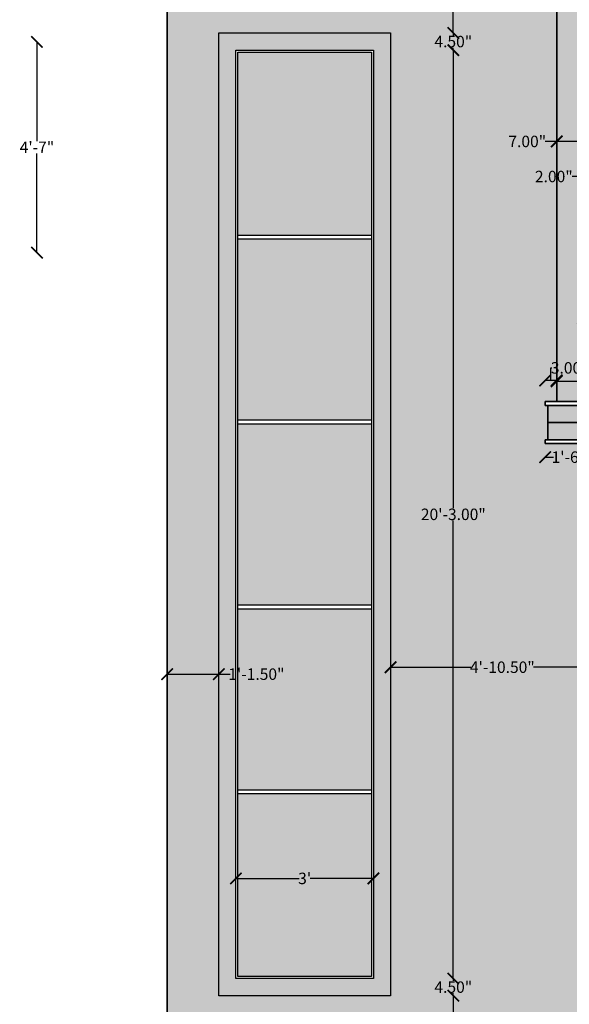
# Model space of a CAD drawing. Units: inches. Extents: x -654 to 390, y -40 to 648.
# Tile 5 of 13: x -40 to 104, y 159 to 417. Entities that reach past the tile are written whole.
import ezdxf

# ---------------------------------------------------------------- set-up
doc = ezdxf.new("R2010")
doc.units = ezdxf.units.IN
doc.header["$PDMODE"] = 3
for name, color, linetype, lineweight in [('A-ANNO-DIMS', 2, 'Continuous', 18), ('A-ELEV', 7, 'Continuous', 35), ('A-ELEV-FILL', 252, 'Continuous', 13), ('A-ELEV-PATT', 8, 'Continuous', 13), ('A-GLAZ', 4, 'Continuous', 25)]:
    doc.layers.add(name, color=color, linetype=linetype, lineweight=lineweight)
doc.styles.get("Standard").update_dxf_attribs({"font": 'arial.ttf'})
doc.dimstyles.get("Standard").update_dxf_attribs({"dimtxt": 3, "dimasz": 3, "dimexe": 0.18, "dimexo": 0.0625, "dimgap": 0.09, "dimtad": 0, "dimtih": 1, "dimtoh": 1, "dimzin": 0, "dimdsep": 46, "dimlunit": 3, "dimtxsty": 'Standard', "dimblk": 'ARCHTICK', "dimcen": 0.09, "dimse1": 1, "dimse2": 1, "dimadec": 0, "dimazin": 0, "dimtfac": 1, "dimtofl": 0, "dimtmove": 0, "dimatfit": 3, "dimfxl": 1, "dimtolj": 1, "dimtzin": 0, "dimarcsym": 0})

# ---------------------------------------------------------------- blocks, each defined once
blk = doc.blocks.new('_ArchTick')
at = {"color": 0, "linetype": 'ByBlock', "const_width": 0.15}
blk.add_lwpolyline([(-0.5, -0.5), (0.5, 0.5)], dxfattribs=at)
blk = doc.blocks.new('*D20')
at = {"layer": 'A-ANNO-DIMS', "color": 0, "lineweight": -2, "transparency": 16777216}
for p, q in [((73.57, 442.63), (73.57, 429.51)), ((73.57, 413.13), (73.57, 426.26))]:
    blk.add_line(p, q, dxfattribs=at)
at = {"layer": 'Defpoints', "color": 0, "transparency": 16777216}
for p in [(73.57, 442.63), (57.15, 413.13), (73.57, 413.13)]:
    blk.add_point(p, dxfattribs=at)
at = {"layer": 'A-ANNO-DIMS', "color": 0, "lineweight": -2, "transparency": 16777216, "xscale": 3, "yscale": 3, "zscale": 3}
for p, rotation in [((73.57, 442.63), 90), ((73.57, 413.13), 270)]:
    blk.add_blockref('_ArchTick', p, dxfattribs=dict(at, rotation=rotation))
at = {"layer": 'A-ANNO-DIMS', "color": 0, "transparency": 16777216, "insert": (73.57, 427.88), "char_height": 3, "attachment_point": 5}
blk.add_mtext('\\A1;2\'-5.50"', dxfattribs=at)
blk = doc.blocks.new('*D21')
at = {"layer": 'A-ANNO-DIMS', "color": 0, "lineweight": -2, "transparency": 16777216}
for p, q in [((73.57, 413.13), (73.57, 412.51)), ((73.57, 408.63), (73.57, 409.26))]:
    blk.add_line(p, q, dxfattribs=at)
at = {"layer": 'Defpoints', "color": 0, "transparency": 16777216}
for p in [(57.15, 413.13), (52.65, 408.63), (73.57, 408.63)]:
    blk.add_point(p, dxfattribs=at)
at = {"layer": 'A-ANNO-DIMS', "color": 0, "lineweight": -2, "transparency": 16777216, "xscale": 3, "yscale": 3, "zscale": 3}
for p, rotation in [((73.57, 413.13), 90), ((73.57, 408.63), 270)]:
    blk.add_blockref('_ArchTick', p, dxfattribs=dict(at, rotation=rotation))
at = {"layer": 'A-ANNO-DIMS', "color": 0, "transparency": 16777216, "insert": (73.57, 410.88), "char_height": 3, "attachment_point": 5}
blk.add_mtext('\\A1;4.50"', dxfattribs=at)
blk = doc.blocks.new('*D22')
at = {"layer": 'A-ANNO-DIMS', "color": 0, "lineweight": -2, "transparency": 16777216}
for p, q in [((73.57, 408.63), (73.57, 288.76)), ((73.57, 165.63), (73.57, 285.51))]:
    blk.add_line(p, q, dxfattribs=at)
at = {"layer": 'Defpoints', "color": 0, "transparency": 16777216}
for p in [(52.65, 408.63), (52.65, 165.63), (73.57, 165.63)]:
    blk.add_point(p, dxfattribs=at)
at = {"layer": 'A-ANNO-DIMS', "color": 0, "lineweight": -2, "transparency": 16777216, "xscale": 3, "yscale": 3, "zscale": 3}
for p, rotation in [((73.57, 408.63), 90), ((73.57, 165.63), 270)]:
    blk.add_blockref('_ArchTick', p, dxfattribs=dict(at, rotation=rotation))
at = {"layer": 'A-ANNO-DIMS', "color": 0, "transparency": 16777216, "insert": (73.57, 287.13), "char_height": 3, "attachment_point": 5}
blk.add_mtext('\\A1;20\'-3.00"', dxfattribs=at)
blk = doc.blocks.new('*D23')
at = {"layer": 'A-ANNO-DIMS', "color": 0, "lineweight": -2, "transparency": 16777216}
for p, q in [((73.57, 165.63), (73.57, 165.01)), ((73.57, 161.13), (73.57, 161.76))]:
    blk.add_line(p, q, dxfattribs=at)
at = {"layer": 'Defpoints', "color": 0, "transparency": 16777216}
for p in [(52.65, 165.63), (57.15, 161.13), (73.57, 161.13)]:
    blk.add_point(p, dxfattribs=at)
at = {"layer": 'A-ANNO-DIMS', "color": 0, "lineweight": -2, "transparency": 16777216, "xscale": 3, "yscale": 3, "zscale": 3}
for p, rotation in [((73.57, 165.63), 90), ((73.57, 161.13), 270)]:
    blk.add_blockref('_ArchTick', p, dxfattribs=dict(at, rotation=rotation))
at = {"layer": 'A-ANNO-DIMS', "color": 0, "transparency": 16777216, "insert": (73.57, 163.38), "char_height": 3, "attachment_point": 5}
blk.add_mtext('\\A1;4.50"', dxfattribs=at)
blk = doc.blocks.new('*D24')
at = {"layer": 'A-ANNO-DIMS', "color": 0, "lineweight": -2, "transparency": 16777216}
for p, q in [((73.57, 161.13), (73.57, 144.76)), ((73.57, 125.13), (73.57, 141.51))]:
    blk.add_line(p, q, dxfattribs=at)
at = {"layer": 'Defpoints', "color": 0, "transparency": 16777216}
for p in [(57.15, 161.13), (73.57, 125.13), (73.57, 125.13)]:
    blk.add_point(p, dxfattribs=at)
at = {"layer": 'A-ANNO-DIMS', "color": 0, "lineweight": -2, "transparency": 16777216, "xscale": 3, "yscale": 3, "zscale": 3}
for p, rotation in [((73.57, 161.13), 90), ((73.57, 125.13), 270)]:
    blk.add_blockref('_ArchTick', p, dxfattribs=dict(at, rotation=rotation))
at = {"layer": 'A-ANNO-DIMS', "color": 0, "transparency": 16777216, "insert": (73.57, 143.13), "char_height": 3, "attachment_point": 5}
blk.add_mtext("\\A1;3'", dxfattribs=at)
blk = doc.blocks.new('*D45')
at = {"layer": 'A-ANNO-DIMS', "color": 0, "lineweight": -2, "transparency": 16777216}
for p, q in [((99.15, 322.17), (99.15, 325.47)), ((99.15, 325.47), (99.33, 325.47)), ((100.65, 322.17), (97.65, 322.17))]:
    blk.add_line(p, q, dxfattribs=at)
at = {"layer": 'Defpoints', "color": 0, "transparency": 16777216}
for p in [(97.65, 322.17), (97.65, 316.63), (100.65, 316.63)]:
    blk.add_point(p, dxfattribs=at)
at = {"layer": 'A-ANNO-DIMS', "color": 0, "lineweight": -2, "transparency": 16777216, "xscale": 3, "yscale": 3, "zscale": 3, "rotation": 180}
blk.add_blockref('_ArchTick', (97.65, 322.17), dxfattribs=at)
at = {"layer": 'A-ANNO-DIMS', "color": 0, "lineweight": -2, "transparency": 16777216, "xscale": 3, "yscale": 3, "zscale": 3}
blk.add_blockref('_ArchTick', (100.65, 322.17), dxfattribs=at)
at = {"layer": 'A-ANNO-DIMS', "color": 0, "transparency": 16777216, "insert": (104.05, 325.47), "char_height": 3, "attachment_point": 5}
blk.add_mtext('\\A1;3.00"', dxfattribs=at)
blk = doc.blocks.new('*D47')
at = {"layer": 'A-ANNO-DIMS', "color": 0, "lineweight": -2, "transparency": 16777216}
for p, q in [((100.65, 321.96), (116.16, 321.96)), ((145.65, 321.96), (130.14, 321.96))]:
    blk.add_line(p, q, dxfattribs=at)
at = {"layer": 'Defpoints', "color": 0, "transparency": 16777216}
for p in [(145.65, 329.63), (100.65, 322.17), (100.65, 321.96)]:
    blk.add_point(p, dxfattribs=at)
at = {"layer": 'A-ANNO-DIMS', "color": 0, "lineweight": -2, "transparency": 16777216, "xscale": 3, "yscale": 3, "zscale": 3, "rotation": 180}
blk.add_blockref('_ArchTick', (100.65, 321.96), dxfattribs=at)
at = {"layer": 'A-ANNO-DIMS', "color": 0, "lineweight": -2, "transparency": 16777216, "xscale": 3, "yscale": 3, "zscale": 3}
blk.add_blockref('_ArchTick', (145.65, 321.96), dxfattribs=at)
at = {"layer": 'A-ANNO-DIMS', "color": 0, "transparency": 16777216, "insert": (123.15, 321.96), "char_height": 3, "attachment_point": 5}
blk.add_mtext('\\A1;3\'-9.00"', dxfattribs=at)
blk = doc.blocks.new('*D48')
at = {"layer": 'A-ANNO-DIMS', "color": 0, "lineweight": -2, "transparency": 16777216}
for p, q in [((113.1, 359.63), (113.1, 339.76)), ((113.1, 316.63), (113.1, 336.51))]:
    blk.add_line(p, q, dxfattribs=at)
at = {"layer": 'Defpoints', "color": 0, "transparency": 16777216}
for p in [(107.65, 359.63), (113.1, 359.63), (100.65, 316.63)]:
    blk.add_point(p, dxfattribs=at)
at = {"layer": 'A-ANNO-DIMS', "color": 0, "lineweight": -2, "transparency": 16777216, "xscale": 3, "yscale": 3, "zscale": 3}
for p, rotation in [((113.1, 359.63), 90), ((113.1, 316.63), 270)]:
    blk.add_blockref('_ArchTick', p, dxfattribs=dict(at, rotation=rotation))
at = {"layer": 'A-ANNO-DIMS', "color": 0, "transparency": 16777216, "insert": (113.1, 338.13), "char_height": 3, "attachment_point": 5}
blk.add_mtext('\\A1;3\'-7.00"', dxfattribs=at)
blk = doc.blocks.new('*D53')
at = {"layer": 'A-ANNO-DIMS', "color": 0, "lineweight": -2, "transparency": 16777216}
for p, q in [((100.65, 384.74), (97.65, 384.74)), ((107.65, 384.74), (100.65, 384.74))]:
    blk.add_line(p, q, dxfattribs=at)
at = {"layer": 'Defpoints', "color": 0, "transparency": 16777216}
for p in [(100.65, 384.74), (100.65, 359.63), (107.65, 359.63)]:
    blk.add_point(p, dxfattribs=at)
at = {"layer": 'A-ANNO-DIMS', "color": 0, "lineweight": -2, "transparency": 16777216, "xscale": 3, "yscale": 3, "zscale": 3, "rotation": 180}
blk.add_blockref('_ArchTick', (100.65, 384.74), dxfattribs=at)
at = {"layer": 'A-ANNO-DIMS', "color": 0, "lineweight": -2, "transparency": 16777216, "xscale": 3, "yscale": 3, "zscale": 3}
blk.add_blockref('_ArchTick', (107.65, 384.74), dxfattribs=at)
at = {"layer": 'A-ANNO-DIMS', "color": 0, "transparency": 16777216, "insert": (92.93, 384.74), "char_height": 3, "attachment_point": 5}
blk.add_mtext('\\A1;7.00"', dxfattribs=at)
blk = doc.blocks.new('*D54')
at = {"layer": 'A-ANNO-DIMS', "color": 0, "lineweight": -2, "transparency": 16777216}
for p, q in [((107.65, 375.56), (104.65, 375.56)), ((109.65, 375.56), (107.65, 375.56))]:
    blk.add_line(p, q, dxfattribs=at)
at = {"layer": 'Defpoints', "color": 0, "transparency": 16777216}
for p in [(107.65, 375.56), (107.65, 361.63), (109.65, 361.63)]:
    blk.add_point(p, dxfattribs=at)
at = {"layer": 'A-ANNO-DIMS', "color": 0, "lineweight": -2, "transparency": 16777216, "xscale": 3, "yscale": 3, "zscale": 3, "rotation": 180}
blk.add_blockref('_ArchTick', (107.65, 375.56), dxfattribs=at)
at = {"layer": 'A-ANNO-DIMS', "color": 0, "lineweight": -2, "transparency": 16777216, "xscale": 3, "yscale": 3, "zscale": 3}
blk.add_blockref('_ArchTick', (109.65, 375.56), dxfattribs=at)
at = {"layer": 'A-ANNO-DIMS', "color": 0, "transparency": 16777216, "insert": (99.89, 375.56), "char_height": 3, "attachment_point": 5}
blk.add_mtext('\\A1;2.00"', dxfattribs=at)
blk = doc.blocks.new('*D65')
at = {"layer": 'A-ANNO-DIMS', "color": 0, "lineweight": -2, "transparency": 16777216}
for p, q in [((-1.35, 245.3), (12.15, 245.3)), ((12.15, 245.3), (15.15, 245.3))]:
    blk.add_line(p, q, dxfattribs=at)
at = {"layer": 'Defpoints', "color": 0, "transparency": 16777216}
for p in [(12.15, 245.3), (12.15, 161.13), (-1.35, 125.13)]:
    blk.add_point(p, dxfattribs=at)
at = {"layer": 'A-ANNO-DIMS', "color": 0, "lineweight": -2, "transparency": 16777216, "xscale": 3, "yscale": 3, "zscale": 3, "rotation": 180}
blk.add_blockref('_ArchTick', (-1.35, 245.3), dxfattribs=at)
at = {"layer": 'A-ANNO-DIMS', "color": 0, "lineweight": -2, "transparency": 16777216, "xscale": 3, "yscale": 3, "zscale": 3}
blk.add_blockref('_ArchTick', (12.15, 245.3), dxfattribs=at)
at = {"layer": 'A-ANNO-DIMS', "color": 0, "transparency": 16777216, "insert": (22, 245.3), "char_height": 3, "attachment_point": 5}
blk.add_mtext('\\A1;1\'-1.50"', dxfattribs=at)
blk = doc.blocks.new('*D66')
at = {"layer": 'A-ANNO-DIMS', "color": 0, "lineweight": -2, "transparency": 16777216}
for p, q in [((16.65, 191.84), (33.18, 191.84)), ((52.65, 191.84), (36.12, 191.84))]:
    blk.add_line(p, q, dxfattribs=at)
at = {"layer": 'Defpoints', "color": 0, "transparency": 16777216}
for p in [(52.65, 191.84), (16.65, 165.63), (52.65, 165.63)]:
    blk.add_point(p, dxfattribs=at)
at = {"layer": 'A-ANNO-DIMS', "color": 0, "lineweight": -2, "transparency": 16777216, "xscale": 3, "yscale": 3, "zscale": 3, "rotation": 180}
blk.add_blockref('_ArchTick', (16.65, 191.84), dxfattribs=at)
at = {"layer": 'A-ANNO-DIMS', "color": 0, "lineweight": -2, "transparency": 16777216, "xscale": 3, "yscale": 3, "zscale": 3}
blk.add_blockref('_ArchTick', (52.65, 191.84), dxfattribs=at)
at = {"layer": 'A-ANNO-DIMS', "color": 0, "transparency": 16777216, "insert": (34.65, 191.84), "char_height": 3, "attachment_point": 5}
blk.add_mtext("\\A1;3'", dxfattribs=at)
blk = doc.blocks.new('*D67')
at = {"layer": 'A-ANNO-DIMS', "color": 0, "lineweight": -2, "transparency": 16777216}
for p, q in [((52.65, 153.11), (57.15, 153.11)), ((57.15, 153.11), (60.15, 153.11))]:
    blk.add_line(p, q, dxfattribs=at)
at = {"layer": 'Defpoints', "color": 0, "transparency": 16777216}
for p in [(52.65, 165.63), (57.15, 161.13), (57.15, 153.11)]:
    blk.add_point(p, dxfattribs=at)
at = {"layer": 'A-ANNO-DIMS', "color": 0, "lineweight": -2, "transparency": 16777216, "xscale": 3, "yscale": 3, "zscale": 3, "rotation": 180}
blk.add_blockref('_ArchTick', (52.65, 153.11), dxfattribs=at)
at = {"layer": 'A-ANNO-DIMS', "color": 0, "lineweight": -2, "transparency": 16777216, "xscale": 3, "yscale": 3, "zscale": 3}
blk.add_blockref('_ArchTick', (57.15, 153.11), dxfattribs=at)
at = {"layer": 'A-ANNO-DIMS', "color": 0, "transparency": 16777216, "insert": (64.93, 153.11), "char_height": 3, "attachment_point": 5}
blk.add_mtext('\\A1;4.50"', dxfattribs=at)
blk = doc.blocks.new('*D68')
at = {"layer": 'A-ANNO-DIMS', "color": 0, "lineweight": -2, "transparency": 16777216}
for p, q in [((12.15, 154.04), (16.65, 154.04)), ((16.65, 154.04), (19.65, 154.04))]:
    blk.add_line(p, q, dxfattribs=at)
at = {"layer": 'Defpoints', "color": 0, "transparency": 16777216}
for p in [(16.65, 165.63), (12.15, 161.13), (16.65, 154.04)]:
    blk.add_point(p, dxfattribs=at)
at = {"layer": 'A-ANNO-DIMS', "color": 0, "lineweight": -2, "transparency": 16777216, "xscale": 3, "yscale": 3, "zscale": 3, "rotation": 180}
blk.add_blockref('_ArchTick', (12.15, 154.04), dxfattribs=at)
at = {"layer": 'A-ANNO-DIMS', "color": 0, "lineweight": -2, "transparency": 16777216, "xscale": 3, "yscale": 3, "zscale": 3}
blk.add_blockref('_ArchTick', (16.65, 154.04), dxfattribs=at)
at = {"layer": 'A-ANNO-DIMS', "color": 0, "transparency": 16777216, "insert": (24.43, 154.04), "char_height": 3, "attachment_point": 5}
blk.add_mtext('\\A1;4.50"', dxfattribs=at)
blk = doc.blocks.new('*D69')
at = {"layer": 'A-ANNO-DIMS', "color": 0, "lineweight": -2, "transparency": 16777216}
for p, q in [((57.15, 247.12), (78.18, 247.12)), ((115.65, 247.12), (94.61, 247.12))]:
    blk.add_line(p, q, dxfattribs=at)
at = {"layer": 'Defpoints', "color": 0, "transparency": 16777216}
for p in [(115.65, 247.12), (115.65, 177.63), (57.15, 161.13)]:
    blk.add_point(p, dxfattribs=at)
at = {"layer": 'A-ANNO-DIMS', "color": 0, "lineweight": -2, "transparency": 16777216, "xscale": 3, "yscale": 3, "zscale": 3, "rotation": 180}
blk.add_blockref('_ArchTick', (57.15, 247.12), dxfattribs=at)
at = {"layer": 'A-ANNO-DIMS', "color": 0, "lineweight": -2, "transparency": 16777216, "xscale": 3, "yscale": 3, "zscale": 3}
blk.add_blockref('_ArchTick', (115.65, 247.12), dxfattribs=at)
at = {"layer": 'A-ANNO-DIMS', "color": 0, "transparency": 16777216, "insert": (86.4, 247.12), "char_height": 3, "attachment_point": 5}
blk.add_mtext('\\A1;4\'-10.50"', dxfattribs=at)
blk = doc.blocks.new('*D70')
at = {"layer": 'A-ANNO-DIMS', "color": 0, "lineweight": -2, "transparency": 16777216}
for p, q in [((97.65, 302.1), (99.8, 302.1)), ((115.65, 302.1), (113.5, 302.1))]:
    blk.add_line(p, q, dxfattribs=at)
at = {"layer": 'Defpoints', "color": 0, "transparency": 16777216}
for p in [(97.65, 305.63), (115.65, 305.63), (115.65, 302.1)]:
    blk.add_point(p, dxfattribs=at)
at = {"layer": 'A-ANNO-DIMS', "color": 0, "lineweight": -2, "transparency": 16777216, "xscale": 3, "yscale": 3, "zscale": 3, "rotation": 180}
blk.add_blockref('_ArchTick', (97.65, 302.1), dxfattribs=at)
at = {"layer": 'A-ANNO-DIMS', "color": 0, "lineweight": -2, "transparency": 16777216, "xscale": 3, "yscale": 3, "zscale": 3}
blk.add_blockref('_ArchTick', (115.65, 302.1), dxfattribs=at)
at = {"layer": 'A-ANNO-DIMS', "color": 0, "transparency": 16777216, "insert": (106.65, 302.1), "char_height": 3, "attachment_point": 5}
blk.add_mtext('\\A1;1\'-6.00"', dxfattribs=at)
blk = doc.blocks.new('*D80')
at = {"layer": 'A-ANNO-DIMS', "color": 0, "lineweight": -2, "transparency": 16777216}
for p, q in [((11.65, 643.23), (25.15, 643.23)), ((25.15, 643.23), (28.15, 643.23))]:
    blk.add_line(p, q, dxfattribs=at)
at = {"layer": 'Defpoints', "color": 0, "transparency": 16777216}
for p in [(25.15, 643.23), (11.65, 20.08), (25.15, 20.08)]:
    blk.add_point(p, dxfattribs=at)
at = {"layer": 'A-ANNO-DIMS', "color": 0, "lineweight": -2, "transparency": 16777216, "xscale": 3, "yscale": 3, "zscale": 3, "rotation": 180}
blk.add_blockref('_ArchTick', (11.65, 643.23), dxfattribs=at)
at = {"layer": 'A-ANNO-DIMS', "color": 0, "lineweight": -2, "transparency": 16777216, "xscale": 3, "yscale": 3, "zscale": 3}
blk.add_blockref('_ArchTick', (25.15, 643.23), dxfattribs=at)
at = {"layer": 'A-ANNO-DIMS', "color": 0, "transparency": 16777216, "insert": (35.58, 643.23), "char_height": 3, "attachment_point": 5}
blk.add_mtext('\\A1;1\'-1 1/2"', dxfattribs=at)
blk = doc.blocks.new('*D101')
at = {"layer": 'A-ANNO-DIMS', "color": 0, "lineweight": -2, "transparency": 16777216}
for p, q in [((-35.45, 410.79), (-35.45, 384.8)), ((-35.45, 355.63), (-35.45, 381.62))]:
    blk.add_line(p, q, dxfattribs=at)
at = {"layer": 'Defpoints', "color": 0, "transparency": 16777216}
for p in [(-35.45, 410.79), (239.87, 410.79), (239.87, 355.63)]:
    blk.add_point(p, dxfattribs=at)
at = {"layer": 'A-ANNO-DIMS', "color": 0, "lineweight": -2, "transparency": 16777216, "xscale": 3, "yscale": 3, "zscale": 3}
for p, rotation in [((-35.45, 410.79), 90), ((-35.45, 355.63), 270)]:
    blk.add_blockref('_ArchTick', p, dxfattribs=dict(at, rotation=rotation))
at = {"layer": 'A-ANNO-DIMS', "color": 0, "transparency": 16777216, "insert": (-35.45, 383.21), "char_height": 3, "attachment_point": 5}
blk.add_mtext('\\A1;4\'-7"', dxfattribs=at)

msp = doc.modelspace()

# ---------------------------------------------------------------- hatches: boundary and pattern name
at = {"layer": 'A-ELEV-FILL'}
h = msp.add_hatch(color=256, dxfattribs=at)
h.dxf.hatch_style = 1
h.paths.add_polyline_path([(115.646, 305.634), (97.646, 305.634), (97.646, 306.634), (98.293, 306.634), (98.293, 315.634), (97.646, 315.634), (97.646, 316.634), (100.646, 316.634), (100.646, 442.634), (-1.354, 442.634), (-1.354, 125.134), (115.646, 125.134)])
h.paths.add_polyline_path([(57.146, 161.134), (12.146, 161.134), (12.146, 413.134), (57.146, 413.134)], flags=16)
h.paths.add_polyline_path([(52.646, 165.634), (16.646, 165.634), (16.646, 408.634), (52.646, 408.634)], flags=0)
h.paths.add_polyline_path([(52.146, 166.134), (17.146, 166.134), (17.146, 408.134), (52.146, 408.134)], flags=0)
h.paths.add_polyline_path([(124.646, 581.134), (-1.354, 581.134), (-1.354, 497.134), (8.646, 497.134), (8.646, 494.634), (12.146, 494.634), (12.146, 546.634), (57.146, 546.634), (57.146, 494.634), (124.646, 494.634)])
h.paths.add_polyline_path([(124.646, 609.134), (-1.354, 609.134), (-1.354, 590.134), (124.646, 590.134)])
h = msp.add_hatch(color=256, dxfattribs=at)
h.dxf.hatch_style = 1
h.paths.add_polyline_path([(346.646, 587.634), (161.035, 587.634), (161.035, 583.634), (342.646, 583.634), (342.646, 497.134), (346.646, 497.134), (346.646, 583.634)])
h.paths.add_polyline_path([(295.646, 315.634), (98.293, 315.634), (98.293, 311.134), (295.646, 311.134)])
h.paths.add_polyline_path([(128.742, 311.134), (98.293, 311.134), (98.293, 306.634), (128.742, 306.634)])
h.paths.add_polyline_path([(140.742, 311.134), (130.742, 311.134), (130.742, 306.634), (140.742, 306.634)])
h.paths.add_polyline_path([(152.742, 311.134), (142.742, 311.134), (142.742, 306.634), (152.742, 306.634)])
h.paths.add_polyline_path([(164.742, 311.134), (154.742, 311.134), (154.742, 306.634), (164.742, 306.634)])
h.paths.add_polyline_path([(176.742, 311.134), (166.742, 311.134), (166.742, 306.634), (176.742, 306.634)])
h.paths.add_polyline_path([(295.646, 311.134), (178.742, 311.134), (178.742, 306.634), (295.646, 306.634)])
h.paths.add_polyline_path([(303.818, 315.634), (295.646, 315.634), (295.646, 311.134), (303.818, 311.134)])
h.paths.add_polyline_path([(303.818, 311.134), (295.646, 311.134), (295.646, 306.634), (303.818, 306.634)])
h = msp.add_hatch(color=256, dxfattribs=at)
h.dxf.hatch_style = 1
h.paths.add_polyline_path([(295.646, 190.634), (178.742, 190.634), (178.742, 177.634), (295.646, 177.634)])
h.paths.add_polyline_path([(176.742, 190.634), (166.742, 190.634), (166.742, 177.634), (176.742, 177.634)])
h.paths.add_polyline_path([(164.742, 190.634), (154.742, 190.634), (154.742, 177.634), (164.742, 177.634)])
h.paths.add_polyline_path([(152.742, 190.634), (142.742, 190.634), (142.742, 177.634), (152.742, 177.634)])
h.paths.add_polyline_path([(140.742, 190.634), (130.742, 190.634), (130.742, 177.634), (140.742, 177.634)])
h.paths.add_polyline_path([(128.742, 190.634), (120.146, 190.634), (120.146, 177.634), (128.742, 177.634)])
h.paths.add_polyline_path([(295.646, 329.634), (145.646, 329.634), (145.646, 442.634), (100.646, 442.634), (100.646, 316.634), (295.646, 316.634)])
h.paths.add_polyline_path([(138.646, 359.634), (107.646, 359.634), (107.646, 438.634), (138.646, 438.634)], flags=16)
h.paths.add_polyline_path([(136.646, 361.634), (109.646, 361.634), (109.646, 436.634), (136.646, 436.634)], flags=0)
h.paths.add_polyline_path([(184.646, 466.634), (7.646, 466.634), (7.646, 453.634), (184.646, 453.634)])
h.paths.add_polyline_path([(184.646, 494.634), (7.646, 494.634), (7.646, 492.634), (184.646, 492.634)])
h.paths.add_polyline_path([(10.336, 492.634), (9.336, 492.634), (9.336, 468.634), (10.336, 468.634)])
h.paths.add_polyline_path([(17.352, 492.634), (16.352, 492.634), (16.352, 468.634), (17.352, 468.634)])
h.paths.add_polyline_path([(24.368, 492.634), (23.368, 492.634), (23.368, 468.634), (24.368, 468.634)])
h.paths.add_polyline_path([(31.384, 492.634), (30.384, 492.634), (30.384, 468.634), (31.384, 468.634)])
h.paths.add_polyline_path([(38.4, 492.634), (37.4, 492.634), (37.4, 468.634), (38.4, 468.634)])
h.paths.add_polyline_path([(45.416, 492.634), (44.416, 492.634), (44.416, 468.634), (45.416, 468.634)])
h.paths.add_polyline_path([(52.432, 492.634), (51.432, 492.634), (51.432, 468.634), (52.432, 468.634)])
h.paths.add_polyline_path([(59.448, 492.634), (58.448, 492.634), (58.448, 468.634), (59.448, 468.634)])
h.paths.add_polyline_path([(66.464, 492.634), (65.464, 492.634), (65.464, 468.634), (66.464, 468.634)])
h.paths.add_polyline_path([(73.48, 492.634), (72.48, 492.634), (72.48, 468.634), (73.48, 468.634)])
h.paths.add_polyline_path([(80.496, 492.634), (79.496, 492.634), (79.496, 468.634), (80.496, 468.634)])
h.paths.add_polyline_path([(87.512, 492.634), (86.512, 492.634), (86.512, 468.634), (87.512, 468.634)])
h.paths.add_polyline_path([(94.528, 492.634), (93.528, 492.634), (93.528, 468.634), (94.528, 468.634)])
h.paths.add_polyline_path([(101.544, 492.634), (100.544, 492.634), (100.544, 468.634), (101.544, 468.634)])
h.paths.add_polyline_path([(108.559, 492.634), (107.559, 492.634), (107.559, 468.634), (108.559, 468.634)])
h.paths.add_polyline_path([(115.575, 492.634), (114.575, 492.634), (114.575, 468.634), (115.575, 468.634)])
h.paths.add_polyline_path([(122.591, 492.634), (121.591, 492.634), (121.591, 468.634), (122.591, 468.634)])
h.paths.add_polyline_path([(129.607, 492.634), (128.607, 492.634), (128.607, 468.634), (129.607, 468.634)])
h.paths.add_polyline_path([(136.623, 492.634), (135.623, 492.634), (135.623, 468.634), (136.623, 468.634)])
h.paths.add_polyline_path([(143.639, 492.634), (142.639, 492.634), (142.639, 468.634), (143.639, 468.634)])
h.paths.add_polyline_path([(150.655, 492.634), (149.655, 492.634), (149.655, 468.634), (150.655, 468.634)])
h.paths.add_polyline_path([(157.671, 492.634), (156.671, 492.634), (156.671, 468.634), (157.671, 468.634)])
h.paths.add_polyline_path([(164.687, 492.634), (163.687, 492.634), (163.687, 468.634), (164.687, 468.634)])
h.paths.add_polyline_path([(171.703, 492.634), (170.703, 492.634), (170.703, 468.634), (171.703, 468.634)])
h.paths.add_polyline_path([(178.719, 492.634), (177.719, 492.634), (177.719, 468.634), (178.719, 468.634)])
h = msp.add_hatch(color=256, dxfattribs=at)
h.dxf.hatch_style = 1
h.paths.add_polyline_path([(60.646, 116.134), (16.396, 116.134), (16.396, 83.134), (18.431, 83.134), (18.431, 113.134), (29.904, 113.134), (29.904, 83.134), (33.082, 83.134), (33.082, 113.134), (44.556, 113.134), (44.556, 83.134), (47.67, 83.134), (47.67, 113.134), (59.143, 113.134), (59.143, 83.134), (60.646, 83.134)])
h.paths.add_polyline_path([(57.146, 413.134), (12.146, 413.134), (12.146, 161.134), (57.146, 161.134)])
h.paths.add_polyline_path([(52.646, 408.634), (52.646, 165.634), (16.646, 165.634), (16.646, 408.634)], flags=16)
h.paths.add_polyline_path([(52.146, 408.134), (52.146, 166.134), (17.146, 166.134), (17.146, 408.134)], flags=0)
at = {"layer": 'A-ELEV-PATT'}
h = msp.add_hatch(dxfattribs=at)
h.set_pattern_fill('GOST_GLASS', color=256)
h.paths.add_polyline_path([(34.168, 540.134), (18.646, 540.134), (18.646, 494.634), (34.168, 494.634)])
h.paths.add_polyline_path([(50.651, 540.134), (35.875, 540.134), (35.875, 494.634), (50.651, 494.634)])
h.paths.add_polyline_path([(23.368, 492.634), (18.646, 492.634), (18.646, 482.634), (23.368, 482.634)])
h.paths.add_polyline_path([(30.384, 492.634), (24.368, 492.634), (24.368, 482.634), (30.384, 482.634)])
h.paths.add_polyline_path([(34.168, 492.634), (31.384, 492.634), (31.384, 482.634), (34.168, 482.634)])
h.paths.add_polyline_path([(44.416, 492.634), (38.4, 492.634), (38.4, 482.634), (44.416, 482.634)])
h.paths.add_polyline_path([(50.651, 492.634), (45.416, 492.634), (45.416, 482.634), (50.651, 482.634)])
h.paths.add_polyline_path([(37.4, 492.634), (35.875, 492.634), (35.875, 482.634), (37.4, 482.634)])
h.paths.add_polyline_path([(52.146, 408.134), (17.146, 408.134), (17.146, 360.234), (52.146, 360.234)])
h.paths.add_polyline_path([(52.146, 359.234), (17.146, 359.234), (17.146, 311.834), (52.146, 311.834)])
h.paths.add_polyline_path([(52.146, 310.834), (17.146, 310.834), (17.146, 263.434), (52.146, 263.434)])
h.paths.add_polyline_path([(52.146, 262.434), (17.146, 262.434), (17.146, 215.034), (52.146, 215.034)])
h.paths.add_polyline_path([(52.146, 214.034), (17.146, 214.034), (17.146, 166.134), (52.146, 166.134)])
h.paths.add_polyline_path([(44.556, 113.134), (33.082, 113.134), (33.082, 83.134), (44.556, 83.134)])
h.paths.add_polyline_path([(29.904, 113.134), (18.431, 113.134), (18.431, 83.134), (29.904, 83.134)])
h.paths.add_polyline_path([(59.143, 113.134), (47.67, 113.134), (47.67, 83.134), (59.143, 83.134)])
h.paths.add_polyline_path([(152.862, 134.63), (137.362, 134.63), (137.362, 74.63), (152.862, 74.63)])
h.paths.add_polyline_path([(170.362, 134.63), (154.862, 134.63), (154.862, 74.63), (170.362, 74.63)])
h.paths.add_polyline_path([(187.858, 134.63), (172.358, 134.63), (172.358, 74.63), (187.858, 74.63)])

# ---------------------------------------------------------------- linework, layer by layer
at = {"layer": 'A-ELEV'}
for p, q in [((-1.354, 89.642), (-1.354, 495.134)), ((100.646, 316.634), (100.646, 442.634)), ((97.646, 316.634), (304.646, 316.634)), ((97.646, 315.634), (97.646, 316.634)), ((97.646, 315.634), (304.646, 315.634)), ((98.293, 315.634), (98.293, 306.634)), ((98.293, 311.134), (303.818, 311.134)), ((97.646, 306.634), (128.742, 306.634)), ((97.646, 305.634), (97.646, 306.634)), ((97.646, 305.634), (128.742, 305.634))]:
    msp.add_line(p, q, dxfattribs=at)
at = {"layer": 'A-GLAZ'}
for p, q in [((17.146, 408.134), (52.146, 408.134)), ((17.146, 166.134), (17.146, 408.134)), ((52.146, 408.134), (52.146, 166.134)), ((17.146, 360.234), (52.146, 360.234)), ((17.146, 359.234), (52.146, 359.234)), ((17.146, 311.834), (52.146, 311.834)), ((17.146, 310.834), (52.146, 310.834)), ((17.146, 263.434), (52.146, 263.434)), ((17.146, 262.434), (52.146, 262.434)), ((17.146, 215.034), (52.146, 215.034)), ((17.146, 214.034), (52.146, 214.034)), ((52.146, 166.134), (17.146, 166.134))]:
    msp.add_line(p, q, dxfattribs=at)
for points in [[(12.146, 413.134), (57.146, 413.134), (57.146, 161.134), (12.146, 161.134)], [(16.646, 408.634), (52.646, 408.634), (52.646, 165.634), (16.646, 165.634)]]:
    msp.add_lwpolyline(points, close=True, dxfattribs=at)

# ---------------------------------------------------------------- dimensions: what is measured, and where the dimension line sits
at = {"layer": 'A-ANNO-DIMS'}
for base, p1, p2, override, picture, middle in [((25.146, 643.234), (11.646, 20.08), (25.146, 20.08), {"dimdec": 1, "dimlfac": 1, "dimrnd": 0, "dimzin": 1, "dimdsep": 46, "dimlunit": 4, "dimfrac": 2}, '*D80', (35.578, 643.234)), ((100.646, 384.745), (107.646, 359.634), (100.646, 359.634), {"dimclrd": 0, "dimclre": 0, "dimclrt": 0}, '*D53', (92.932, 384.745)), ((107.646, 375.564), (109.646, 361.634), (107.646, 361.634), {"dimclrd": 0, "dimclre": 0, "dimclrt": 0}, '*D54', (99.894, 375.564)), ((97.646, 322.175), (100.646, 316.634), (97.646, 316.634), {"dimclrd": 0, "dimclre": 0, "dimclrt": 0, "dimtmove": 1}, '*D45', (99.416, 325.465)), ((100.646, 321.96), (145.646, 329.634), (100.646, 322.175), {"dimclrd": 0, "dimclre": 0, "dimclrt": 0, "dimtmove": 1}, '*D47', (123.146, 321.96)), ((115.646, 302.096), (97.646, 305.634), (115.646, 305.634), {"dimclrd": 0, "dimclre": 0, "dimclrt": 0}, '*D70', (106.646, 302.096)), ((115.646, 247.118), (57.146, 161.134), (115.646, 177.634), {"dimclrd": 0, "dimclre": 0, "dimclrt": 0}, '*D69', (86.396, 247.118)), ((12.146, 245.302), (-1.354, 125.134), (12.146, 161.134), {"dimclrd": 0, "dimclre": 0, "dimclrt": 0}, '*D65', (21.996, 245.302)), ((52.646, 191.835), (16.646, 165.634), (52.646, 165.634), {"dimclrd": 0, "dimclre": 0, "dimclrt": 0}, '*D66', (34.646, 191.835)), ((16.646, 154.036), (12.146, 161.134), (16.646, 165.634), {"dimclrd": 0, "dimclre": 0, "dimclrt": 0}, '*D68', (24.434, 154.036)), ((57.146, 153.11), (52.646, 165.634), (57.146, 161.134), {"dimclrd": 0, "dimclre": 0, "dimclrt": 0}, '*D67', (64.934, 153.11))]:
    dim = msp.add_linear_dim(base=base, p1=p1, p2=p2, dimstyle='Standard', override=override, dxfattribs=at)
    dim.commit()
    dim.dimension.update_dxf_attribs({"geometry": picture, "text_midpoint": middle})
for base, p1, p2, override, picture, middle in [((73.566, 413.134), (73.566, 442.634), (57.146, 413.134), {"dimclrd": 0, "dimclre": 0, "dimclrt": 0, "dimtmove": 1}, '*D20', (73.566, 427.884)), ((-35.454, 410.786), (239.871, 355.634), (239.871, 410.786), {"dimdec": 1, "dimlfac": 1, "dimrnd": 0, "dimzin": 1, "dimdsep": 46, "dimlunit": 4, "dimfrac": 2}, '*D101', (-35.454, 383.21)), ((73.566, 408.634), (57.146, 413.134), (52.646, 408.634), {"dimclrd": 0, "dimclre": 0, "dimclrt": 0, "dimtmove": 1}, '*D21', (73.566, 410.884)), ((73.566, 165.634), (52.646, 408.634), (52.646, 165.634), {"dimclrd": 0, "dimclre": 0, "dimclrt": 0, "dimtmove": 1}, '*D22', (73.566, 287.134)), ((113.102, 359.634), (100.646, 316.634), (107.646, 359.634), {"dimclrd": 0, "dimclre": 0, "dimclrt": 0}, '*D48', (113.102, 338.134)), ((73.566, 161.134), (52.646, 165.634), (57.146, 161.134), {"dimclrd": 0, "dimclre": 0, "dimclrt": 0, "dimtmove": 1}, '*D23', (73.566, 163.384)), ((73.566, 125.134), (57.146, 161.134), (73.566, 125.134), {"dimclrd": 0, "dimclre": 0, "dimclrt": 0, "dimtmove": 1}, '*D24', (73.566, 143.134))]:
    dim = msp.add_linear_dim(base=base, p1=p1, p2=p2, angle=90, dimstyle='Standard', override=override, dxfattribs=at)
    dim.commit()
    dim.dimension.update_dxf_attribs({"geometry": picture, "text_midpoint": middle})

doc.saveas('drawing.dxf')
